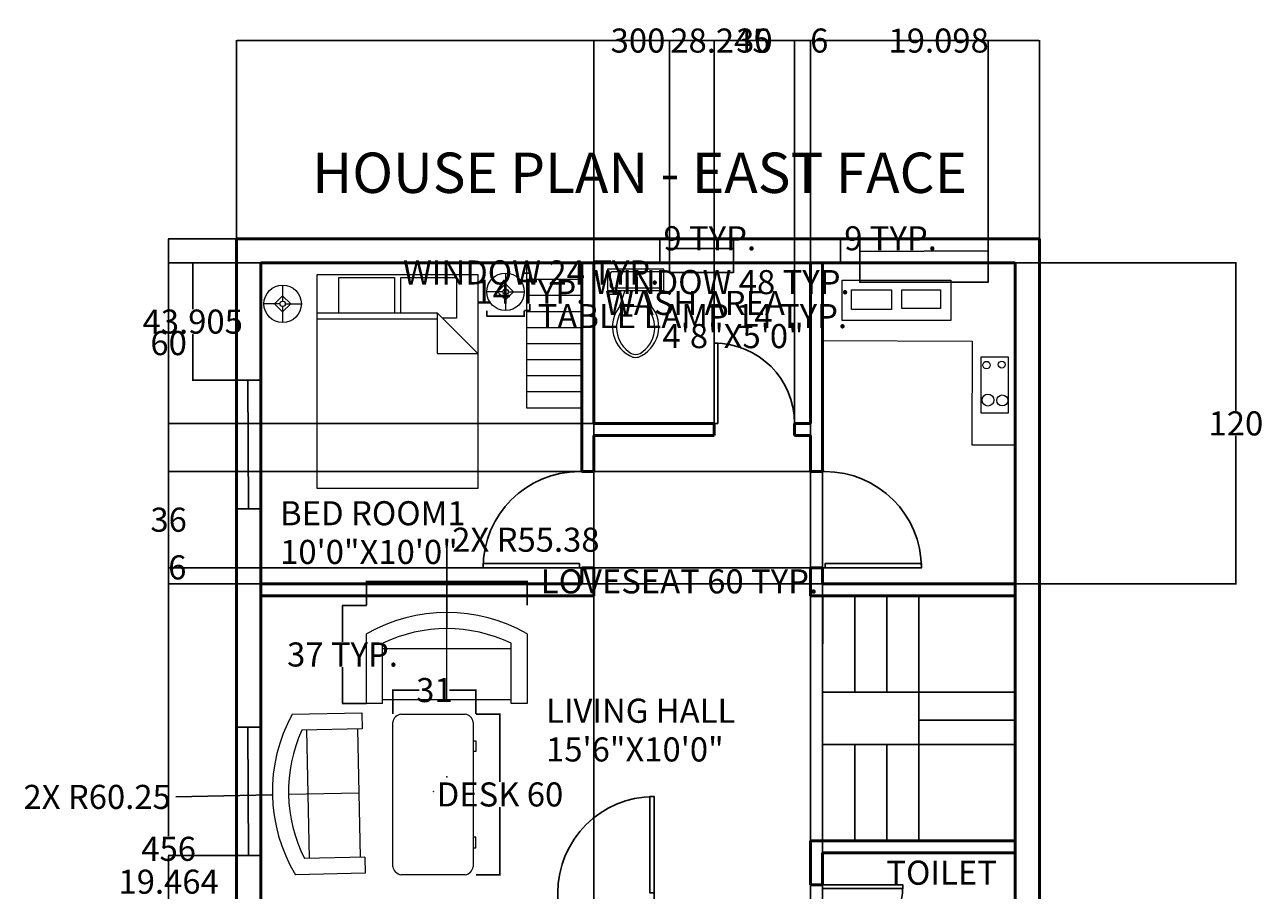
# Model space of a CAD drawing. Units: inches. Extents: x -49 to 419, y 83 to 650.
# Tile 2 of 2: x -49 to 414, y 327 to 650. Entities that reach past the tile are written whole.
import ezdxf

# ---------------------------------------------------------------- set-up
doc = ezdxf.new("R2010")
doc.units = ezdxf.units.IN
for name, color, linetype, lineweight in [('A-ANNO-DIMS', 2, 'Continuous', 18), ('A-ANNO-TEXT', 2, 'Continuous', 35), ('A-AREA-IDEN', 2, 'Continuous', 25), ('A-DOOR', 20, 'Continuous', 25), ('A-EQPM', 130, 'Continuous', 18), ('A-FLOR-CASE', 130, 'Continuous', 18), ('A-FLOR-FIXT', 130, 'Continuous', 18), ('A-FLOR-STRS', 150, 'Continuous', 25), ('A-GLAZ', 70, 'Continuous', 25), ('FUR', 130, 'Continuous', 18), ('WAL', 210, 'Continuous', 50)]:
    doc.layers.add(name, color=color, linetype=linetype, lineweight=lineweight)
doc.styles.get("Standard").update_dxf_attribs({"font": 'arial.ttf', "height": 9})
doc.dimstyles.get("Standard").update_dxf_attribs({"dimtxt": 0.18, "dimasz": 0.18, "dimexe": 0.18, "dimexo": 0.0625, "dimgap": 0.09, "dimtad": 0, "dimtih": 1, "dimtoh": 1, "dimdec": 4, "dimzin": 0, "dimdsep": 46, "dimtxsty": 'Standard', "dimcen": 0.09, "dimadec": 0, "dimazin": 0, "dimtfac": 1, "dimtdec": 4, "dimtofl": 0, "dimtmove": 0, "dimatfit": 3, "dimfxl": 1, "dimtolj": 1, "dimtzin": 0, "dimarcsym": 0})

# ---------------------------------------------------------------- blocks, each defined once
blk = doc.blocks.new('*U2')
for p, q in [((0, 0), (0, -6)), ((40, 0), (40, -6))]:
    blk.add_line(p, q)
blk.add_lwpolyline([(0, 0), (0, 40), (1.75, 40), (1.75, 0)], close=True)
blk.add_arc((0, 0), 40, 0, 90)
blk = doc.blocks.new('*U4')
for p, q in [((9.5, -6), (9.5, -2)), ((-10, -8.5), (-8, -8.5)), ((-10, -9.5), (-10, -8.5)), ((-8, -8.5), (-8, -8)), ((-7, -8), (-7, -9.5)), ((-4, -8), (-6, -14)), ((4, -8), (6, -14)), ((-7, -9.5), (-10, -9.5)), ((4, -14), (-4, -14))]:
    blk.add_line(p, q)
blk.add_lwpolyline([(10.5, -8), (10.5, 0), (-10.5, 0), (-10.5, -8)], close=True)
for points in [[(-9.5, -2), (-9.5, -6)], [(8.5, -1), (-8.5, -1)], [(-8.5, -7), (8.5, -7)]]:
    blk.add_lwpolyline(points)
for centre, radius, start, end in [((-8.62, -1.88), 0.884, 81.8699, 188.1301), ((8.62, -1.88), 0.884, 351.8699, 98.1301), ((-8.62, -6.12), 0.884, 171.8699, 278.1301), ((8.62, -6.12), 0.884, 261.8699, 8.1301), ((3.52, -21.58), 12.17, 141.4691, 247.9714), ((4.2, -21.82), 11.33, 136.3677, 238.9468), ((-3.52, -21.58), 12.17, 292.0284, 38.5307), ((-4.2, -21.82), 11.33, 301.053, 43.6321), ((0, -27.88), 4, 245.7318, 294.2682), ((0, -29), 4, 254.8605, 285.1395)]:
    blk.add_arc(centre, radius, start, end)
blk = doc.blocks.new('Bed - Queen')
for p, q in [((0, -80.00003), (0, 0)), ((0, 0), (59.99999, 0)), ((59.99999, 0), (59.99999, -80.00003)), ((7.99999, -1.2), (28.79998, -1.2)), ((7.99999, -14.4), (7.99999, -1.2)), ((28.79998, -1.2), (28.79998, -14.4)), ((31.19999, -1.2), (51.99999, -1.2)), ((31.19999, -14.4), (31.19999, -1.2)), ((51.99999, -1.2), (51.99999, -16.4)), ((0, -14.4), (44.8, -14.4)), ((44.8, -16.8), (0, -16.8)), ((59.99999, -29.6), (44.8, -14.4)), ((44.8, -14.4), (44.8, -29.6)), ((51.99999, -16.4), (46.79936, -16.4)), ((44.8, -29.6), (59.99999, -29.6)), ((59.99999, -80.00003), (0, -80.00003))]:
    blk.add_line(p, q)
blk = doc.blocks.new('Lamp - Table')
for p, q in [((0, 7), (0, 1)), ((-1, 0), (-7, 0)), ((0, 3), (-3, 0)), ((-3, 0), (0, -3)), ((3, 0), (0, 3)), ((0, -3), (3, 0)), ((1, 0), (7, 0)), ((0, -1), (0, -7))]:
    blk.add_line(p, q)
for radius in [7, 1]:
    blk.add_circle((0, 0), radius)
blk = doc.blocks.new('Desk - 30 x 60 in.')
for p, q in [((-26.999995, 0), (26.999995, 0)), ((-29.999995, -27), (-29.999995, -3)), ((29.999995, -3), (29.999995, -27)), ((26.999995, -30), (-26.999995, -30)), ((-20.000005, -30), (-20.000005, -31)), ((-20.000005, -31), (-16.000005, -31)), ((-16.000005, -31), (-16.000005, -30)), ((15.999995, -31), (15.999995, -30)), ((19.999995, -31), (15.999995, -31)), ((19.999995, -30), (19.999995, -31))]:
    blk.add_line(p, q)
for centre, start, end in [((-26.499995, -3.5), 98.1301, 171.8699), ((26.499995, -3.5), 8.130102, 81.8699), ((-26.499995, -26.5), 188.1301, 261.8699), ((26.499995, -26.5), 278.1301, 351.8699)]:
    blk.add_arc(centre, 3.535534, start, end)
blk = doc.blocks.new('Sofa - Roundback Loveseat 5 ft.')
for p, q in [((0, -32.44198), (0, -5.99998)), ((-24, -33.99998), (-24, -11.46958)), ((-23.9998, -13.38178), (23.99986, -13.38178)), ((24.00004, -33.99998), (24.00004, -11.46958)), ((-24, -32.44198), (24.00004, -32.44198))]:
    blk.add_line(p, q)
for points in [[(-24, -33.99998), (-30, -33.99998), (-30, -7.99998)], [(30.00004, -7.99998), (30.00004, -33.99998), (24.00004, -33.99998)]]:
    blk.add_lwpolyline(points)
for centre, radius, start, end in [((0, -60.24998), 60.24998, 60.13715, 119.8628), ((0, -61.38438), 55.38444, 64.32083, 115.6792)]:
    blk.add_arc(centre, radius, start, end)
blk = doc.blocks.new('WIN-48IN')
for p, q in [((0, 48), (0, 0)), ((9, 48), (0, 48)), ((4.19, 48), (4.5, 0)), ((9, 0), (9, 48)), ((0, 0), (9, 0))]:
    blk.add_line(p, q)
blk = doc.blocks.new('WIN-24IN')
for p, q in [((0, 24), (0, 0)), ((9, 24), (0, 24)), ((0, 24), (5.33, 24)), ((5.33, 24), (5.33, 0)), ((9, 0), (9, 24)), ((0, 0), (9, 0))]:
    blk.add_line(p, q)
blk = doc.blocks.new('*D14')
at = {"layer": 'A-ANNO-DIMS', "color": 0, "lineweight": -2, "transparency": 16777216}
for p, q in [((262.9, 560.94), (262.9, 553.62)), ((310.9, 560.94), (310.9, 553.62)), ((262.9, 553.8), (262.72, 553.8)), ((310.72, 553.8), (263.08, 553.8))]:
    blk.add_line(p, q, dxfattribs=at)
at = {"layer": 'A-ANNO-DIMS', "color": 0, "transparency": 16777216}
for points in [[(263.08, 553.83), (263.08, 553.77), (262.9, 553.8)], [(310.72, 553.83), (310.72, 553.77), (310.9, 553.8)]]:
    blk.add_solid(points, dxfattribs=at)
at = {"layer": 'Defpoints', "color": 0, "transparency": 16777216}
for p in [(262.9, 561), (310.9, 561), (262.9, 553.8)]:
    blk.add_point(p, dxfattribs=at)
at = {"layer": 'A-ANNO-DIMS', "color": 0, "transparency": 16777216, "insert": (211.21, 553.8), "char_height": 9, "attachment_point": 5}
blk.add_mtext('\\A1;WINDOW 48 TYP.', dxfattribs=at)
blk = doc.blocks.new('*D15')
at = {"layer": 'A-ANNO-DIMS', "color": 0, "lineweight": -2, "transparency": 16777216}
for p, q in [((262.84, 570), (255.52, 570)), ((255.7, 570), (255.7, 570.18)), ((255.7, 570.18), (255.88, 570.18)), ((255.7, 561.18), (255.7, 569.82)), ((262.84, 561), (255.52, 561))]:
    blk.add_line(p, q, dxfattribs=at)
at = {"layer": 'A-ANNO-DIMS', "color": 0, "transparency": 16777216}
for points in [[(255.67, 569.82), (255.73, 569.82), (255.7, 570)], [(255.67, 561.18), (255.73, 561.18), (255.7, 561)]]:
    blk.add_solid(points, dxfattribs=at)
at = {"layer": 'Defpoints', "color": 0, "transparency": 16777216}
for p in [(255.7, 570), (262.9, 570), (262.9, 561)]:
    blk.add_point(p, dxfattribs=at)
at = {"layer": 'A-ANNO-DIMS', "color": 0, "transparency": 16777216, "insert": (274.38, 570.18), "char_height": 9, "attachment_point": 5}
blk.add_mtext('\\A1;9 TYP.', dxfattribs=at)
blk = doc.blocks.new('*D16')
at = {"layer": 'A-ANNO-DIMS', "color": 0, "lineweight": -2, "transparency": 16777216}
for p, q in [((191.74, 560.94), (191.74, 557.22)), ((215.74, 560.94), (215.74, 557.22)), ((191.74, 557.4), (191.56, 557.4)), ((215.56, 557.4), (191.92, 557.4))]:
    blk.add_line(p, q, dxfattribs=at)
at = {"layer": 'A-ANNO-DIMS', "color": 0, "transparency": 16777216}
for points in [[(191.92, 557.43), (191.92, 557.37), (191.74, 557.4)], [(215.56, 557.43), (215.56, 557.37), (215.74, 557.4)]]:
    blk.add_solid(points, dxfattribs=at)
at = {"layer": 'Defpoints', "color": 0, "transparency": 16777216}
for p in [(191.74, 561), (215.74, 561), (191.74, 557.4)]:
    blk.add_point(p, dxfattribs=at)
at = {"layer": 'A-ANNO-DIMS', "color": 0, "transparency": 16777216, "insert": (140.06, 557.4), "char_height": 9, "attachment_point": 5}
blk.add_mtext('\\A1;WINDOW 24 TYP.', dxfattribs=at)
blk = doc.blocks.new('*D17')
at = {"layer": 'A-ANNO-DIMS', "color": 0, "lineweight": -2, "transparency": 16777216}
for p, q in [((191.68, 570), (187.96, 570)), ((188.14, 570), (188.14, 570.18)), ((188.14, 570.18), (188.32, 570.18)), ((188.14, 561.18), (188.14, 569.82)), ((191.68, 561), (187.96, 561))]:
    blk.add_line(p, q, dxfattribs=at)
at = {"layer": 'A-ANNO-DIMS', "color": 0, "transparency": 16777216}
for points in [[(188.11, 569.82), (188.17, 569.82), (188.14, 570)], [(188.11, 561.18), (188.17, 561.18), (188.14, 561)]]:
    blk.add_solid(points, dxfattribs=at)
at = {"layer": 'Defpoints', "color": 0, "transparency": 16777216}
for p in [(188.14, 570), (191.74, 570), (191.74, 561)]:
    blk.add_point(p, dxfattribs=at)
at = {"layer": 'A-ANNO-DIMS', "color": 0, "transparency": 16777216, "insert": (206.82, 570.18), "char_height": 9, "attachment_point": 5}
blk.add_mtext('\\A1;9 TYP.', dxfattribs=at)
blk = doc.blocks.new('*D20')
at = {"layer": 'A-ANNO-DIMS', "color": 0, "lineweight": -2, "transparency": 16777216}
for p, q in [((123.51, 543.12), (123.51, 540.91)), ((137.51, 543.12), (137.51, 540.91)), ((123.69, 541.09), (137.33, 541.09)), ((137.51, 541.09), (137.69, 541.09))]:
    blk.add_line(p, q, dxfattribs=at)
at = {"layer": 'A-ANNO-DIMS', "color": 0, "transparency": 16777216}
for points in [[(123.69, 541.12), (123.69, 541.06), (123.51, 541.09)], [(137.33, 541.12), (137.33, 541.06), (137.51, 541.09)]]:
    blk.add_solid(points, dxfattribs=at)
at = {"layer": 'Defpoints', "color": 0, "transparency": 16777216}
for p in [(123.51, 543.19), (137.51, 543.19), (137.51, 541.09)]:
    blk.add_point(p, dxfattribs=at)
at = {"layer": 'A-ANNO-DIMS', "color": 0, "transparency": 16777216, "insert": (200.33, 541.09), "char_height": 9, "attachment_point": 5}
blk.add_mtext('\\A1;TABLE LAMP 14 TYP.', dxfattribs=at)
blk = doc.blocks.new('*D21')
at = {"layer": 'A-ANNO-DIMS', "color": 0, "lineweight": -2, "transparency": 16777216}
for p, q in [((137.57, 557.19), (139.79, 557.19)), ((139.61, 557.01), (139.61, 554.8)), ((137.57, 543.19), (139.79, 543.19)), ((139.61, 543.37), (139.61, 545.57))]:
    blk.add_line(p, q, dxfattribs=at)
at = {"layer": 'A-ANNO-DIMS', "color": 0, "transparency": 16777216}
for points in [[(139.58, 557.01), (139.64, 557.01), (139.61, 557.19)], [(139.58, 543.37), (139.64, 543.37), (139.61, 543.19)]]:
    blk.add_solid(points, dxfattribs=at)
at = {"layer": 'Defpoints', "color": 0, "transparency": 16777216}
for p in [(137.51, 557.19), (139.61, 557.19), (137.51, 543.19)]:
    blk.add_point(p, dxfattribs=at)
at = {"layer": 'A-ANNO-DIMS', "color": 0, "transparency": 16777216, "insert": (139.61, 550.19), "char_height": 9, "attachment_point": 5}
blk.add_mtext('\\A1;14 TYP.', dxfattribs=at)
blk = doc.blocks.new('*D22')
at = {"layer": 'A-ANNO-DIMS', "color": 0, "lineweight": -2, "transparency": 16777216}
for p, q in [((78.58, 433.02), (78.58, 442.14)), ((78.76, 441.96), (138.4, 441.96)), ((138.58, 433.02), (138.58, 442.14)), ((138.58, 441.96), (138.76, 441.96))]:
    blk.add_line(p, q, dxfattribs=at)
at = {"layer": 'A-ANNO-DIMS', "color": 0, "transparency": 16777216}
for points in [[(78.76, 441.99), (78.76, 441.93), (78.58, 441.96)], [(138.4, 441.99), (138.4, 441.93), (138.58, 441.96)]]:
    blk.add_solid(points, dxfattribs=at)
at = {"layer": 'Defpoints', "color": 0, "transparency": 16777216}
for p in [(138.58, 441.96), (78.58, 432.96), (138.58, 432.96)]:
    blk.add_point(p, dxfattribs=at)
at = {"layer": 'A-ANNO-DIMS', "color": 0, "transparency": 16777216, "insert": (195.49, 441.96), "char_height": 9, "attachment_point": 5}
blk.add_mtext('\\A1;LOVESEAT 60 TYP.', dxfattribs=at)
blk = doc.blocks.new('*D23')
at = {"layer": 'A-ANNO-DIMS', "color": 0, "lineweight": -2, "transparency": 16777216}
for p, q in [((78.52, 432.96), (69.4, 432.96)), ((69.58, 432.78), (69.58, 419.32)), ((69.58, 396.48), (69.58, 409.94)), ((78.52, 396.3), (69.4, 396.3))]:
    blk.add_line(p, q, dxfattribs=at)
at = {"layer": 'A-ANNO-DIMS', "color": 0, "transparency": 16777216}
for points in [[(69.55, 432.78), (69.61, 432.78), (69.58, 432.96)], [(69.55, 396.48), (69.61, 396.48), (69.58, 396.3)]]:
    blk.add_solid(points, dxfattribs=at)
at = {"layer": 'Defpoints', "color": 0, "transparency": 16777216}
for p in [(69.58, 432.96), (78.58, 432.96), (78.58, 396.3)]:
    blk.add_point(p, dxfattribs=at)
at = {"layer": 'A-ANNO-DIMS', "color": 0, "transparency": 16777216, "insert": (69.58, 414.63), "char_height": 9, "attachment_point": 5}
blk.add_mtext('\\A1;37 TYP.', dxfattribs=at)
blk = doc.blocks.new('*D24')
at = {"layer": 'A-ANNO-DIMS', "color": 0, "lineweight": -2, "transparency": 16777216}
for p, q in [((119.49, 392.33), (128.6, 392.33)), ((128.42, 392.15), (128.42, 367.08)), ((128.42, 332.51), (128.42, 357.59)), ((119.49, 332.33), (128.6, 332.33))]:
    blk.add_line(p, q, dxfattribs=at)
at = {"layer": 'A-ANNO-DIMS', "color": 0, "transparency": 16777216}
for points in [[(128.39, 392.15), (128.45, 392.15), (128.42, 392.33)], [(128.39, 332.51), (128.45, 332.51), (128.42, 332.33)]]:
    blk.add_solid(points, dxfattribs=at)
at = {"layer": 'Defpoints', "color": 0, "transparency": 16777216}
for p in [(119.42, 392.33), (128.42, 392.33), (119.42, 332.33)]:
    blk.add_point(p, dxfattribs=at)
at = {"layer": 'A-ANNO-DIMS', "color": 0, "transparency": 16777216, "insert": (128.42, 362.33), "char_height": 9, "attachment_point": 5}
blk.add_mtext('\\A1;DESK 60', dxfattribs=at)
blk = doc.blocks.new('*D25')
at = {"layer": 'A-ANNO-DIMS', "color": 0, "lineweight": -2, "transparency": 16777216}
for p, q in [((88.42, 392.4), (88.42, 401.51)), ((88.6, 401.33), (98.26, 401.33)), ((119.24, 401.33), (109.59, 401.33)), ((119.42, 392.4), (119.42, 401.51))]:
    blk.add_line(p, q, dxfattribs=at)
at = {"layer": 'A-ANNO-DIMS', "color": 0, "transparency": 16777216}
for points in [[(88.6, 401.36), (88.6, 401.3), (88.42, 401.33)], [(119.24, 401.36), (119.24, 401.3), (119.42, 401.33)]]:
    blk.add_solid(points, dxfattribs=at)
at = {"layer": 'Defpoints', "color": 0, "transparency": 16777216}
for p in [(88.42, 401.33), (88.42, 392.33), (119.42, 392.33)]:
    blk.add_point(p, dxfattribs=at)
at = {"layer": 'A-ANNO-DIMS', "color": 0, "transparency": 16777216, "insert": (103.92, 401.33), "char_height": 9, "attachment_point": 5}
blk.add_mtext('\\A1;31', dxfattribs=at)
blk = doc.blocks.new('*D26')
at = {"layer": 'A-ANNO-DIMS', "color": 0, "lineweight": -2, "transparency": 16777216}
for p, q in [((30, 570.06), (30, 644.25)), ((30.18, 644.07), (169.99, 644.07)), ((329.82, 644.07), (190.01, 644.07)), ((330, 570.06), (330, 644.25))]:
    blk.add_line(p, q, dxfattribs=at)
at = {"layer": 'A-ANNO-DIMS', "color": 0, "transparency": 16777216}
for points in [[(30.18, 644.1), (30.18, 644.04), (30, 644.07)], [(329.82, 644.1), (329.82, 644.04), (330, 644.07)]]:
    blk.add_solid(points, dxfattribs=at)
at = {"layer": 'Defpoints', "color": 0, "transparency": 16777216}
for p in [(330, 644.07), (30, 570), (330, 570)]:
    blk.add_point(p, dxfattribs=at)
at = {"layer": 'A-ANNO-DIMS', "color": 0, "transparency": 16777216, "insert": (180, 644.07), "char_height": 9, "attachment_point": 5}
blk.add_mtext('\\A1;300', dxfattribs=at)
blk = doc.blocks.new('*D27')
at = {"layer": 'A-ANNO-DIMS', "color": 0, "lineweight": -2, "transparency": 16777216}
for p, q in [((29.94, 570), (4.42, 570)), ((4.6, 569.82), (4.6, 346.69)), ((4.6, 114.18), (4.6, 337.31)), ((29.94, 114), (4.42, 114))]:
    blk.add_line(p, q, dxfattribs=at)
at = {"layer": 'A-ANNO-DIMS', "color": 0, "transparency": 16777216}
for points in [[(4.57, 569.82), (4.63, 569.82), (4.6, 570)], [(4.57, 114.18), (4.63, 114.18), (4.6, 114)]]:
    blk.add_solid(points, dxfattribs=at)
at = {"layer": 'Defpoints', "color": 0, "transparency": 16777216}
for p in [(4.6, 570), (30, 570), (30, 114)]:
    blk.add_point(p, dxfattribs=at)
at = {"layer": 'A-ANNO-DIMS', "color": 0, "transparency": 16777216, "insert": (4.6, 342), "char_height": 9, "attachment_point": 5}
blk.add_mtext('\\A1;456', dxfattribs=at)
blk = doc.blocks.new('*D30')
at = {"layer": 'A-ANNO-DIMS', "color": 0, "lineweight": -2, "transparency": 16777216}
for p, q in [((29.94, 339.46), (4.42, 339.46)), ((4.6, 339.28), (4.6, 334.42)), ((4.6, 320.18), (4.6, 325.05)), ((38.94, 320), (4.42, 320))]:
    blk.add_line(p, q, dxfattribs=at)
at = {"layer": 'A-ANNO-DIMS', "color": 0, "transparency": 16777216}
for points in [[(4.57, 339.28), (4.63, 339.28), (4.6, 339.46)], [(4.57, 320.18), (4.63, 320.18), (4.6, 320)]]:
    blk.add_solid(points, dxfattribs=at)
at = {"layer": 'Defpoints', "color": 0, "transparency": 16777216}
for p in [(30, 339.46), (4.6, 320), (39, 320)]:
    blk.add_point(p, dxfattribs=at)
at = {"layer": 'A-ANNO-DIMS', "color": 0, "transparency": 16777216, "insert": (4.6, 329.73), "char_height": 9, "attachment_point": 5}
blk.add_mtext('\\A1;19.464', dxfattribs=at)
blk = doc.blocks.new('*D31')
at = {"layer": 'A-ANNO-DIMS', "color": 0, "lineweight": -2, "transparency": 16777216}
for p, q in [((38.94, 561), (13.42, 561)), ((13.6, 560.82), (13.6, 543.74)), ((13.6, 517.27), (13.6, 534.36)), ((38.94, 517.09), (13.42, 517.09))]:
    blk.add_line(p, q, dxfattribs=at)
at = {"layer": 'A-ANNO-DIMS', "color": 0, "transparency": 16777216}
for points in [[(13.57, 560.82), (13.63, 560.82), (13.6, 561)], [(13.57, 517.27), (13.63, 517.27), (13.6, 517.09)]]:
    blk.add_solid(points, dxfattribs=at)
at = {"layer": 'Defpoints', "color": 0, "transparency": 16777216}
for p in [(13.6, 561), (39, 561), (39, 517.09)]:
    blk.add_point(p, dxfattribs=at)
at = {"layer": 'A-ANNO-DIMS', "color": 0, "transparency": 16777216, "insert": (13.6, 539.05), "char_height": 9, "attachment_point": 5}
blk.add_mtext('\\A1;43.905', dxfattribs=at)
blk = doc.blocks.new('*D32')
at = {"layer": 'A-ANNO-DIMS', "color": 0, "lineweight": -2, "transparency": 16777216}
for p, q in [((163.5, 561.06), (163.5, 644.25)), ((163.68, 644.07), (191.56, 644.07)), ((191.74, 561.06), (191.74, 644.25)), ((191.74, 644.07), (191.92, 644.07))]:
    blk.add_line(p, q, dxfattribs=at)
at = {"layer": 'A-ANNO-DIMS', "color": 0, "transparency": 16777216}
for points in [[(163.68, 644.1), (163.68, 644.04), (163.5, 644.07)], [(191.56, 644.1), (191.56, 644.04), (191.74, 644.07)]]:
    blk.add_solid(points, dxfattribs=at)
at = {"layer": 'Defpoints', "color": 0, "transparency": 16777216}
for p in [(191.74, 644.07), (163.5, 561), (191.74, 561)]:
    blk.add_point(p, dxfattribs=at)
at = {"layer": 'A-ANNO-DIMS', "color": 0, "transparency": 16777216, "insert": (210.81, 644.07), "char_height": 9, "attachment_point": 5}
blk.add_mtext('\\A1;28.245', dxfattribs=at)
blk = doc.blocks.new('*D33')
at = {"layer": 'A-ANNO-DIMS', "color": 0, "lineweight": -2, "transparency": 16777216}
for p, q in [((310.9, 644.07), (310.72, 644.07)), ((310.9, 570.06), (310.9, 644.25)), ((329.82, 644.07), (311.08, 644.07)), ((330, 570.06), (330, 644.25))]:
    blk.add_line(p, q, dxfattribs=at)
at = {"layer": 'A-ANNO-DIMS', "color": 0, "transparency": 16777216}
for points in [[(311.08, 644.1), (311.08, 644.04), (310.9, 644.07)], [(329.82, 644.1), (329.82, 644.04), (330, 644.07)]]:
    blk.add_solid(points, dxfattribs=at)
at = {"layer": 'Defpoints', "color": 0, "transparency": 16777216}
for p in [(310.9, 644.07), (310.9, 570), (330, 570)]:
    blk.add_point(p, dxfattribs=at)
at = {"layer": 'A-ANNO-DIMS', "color": 0, "transparency": 16777216, "insert": (292.36, 644.07), "char_height": 9, "attachment_point": 5}
blk.add_mtext('\\A1;19.098', dxfattribs=at)
blk = doc.blocks.new('*D36')
at = {"layer": 'A-ANNO-DIMS', "color": 0, "lineweight": -2, "transparency": 16777216}
for p, q in [((163.5, 500.94), (163.5, 88.42)), ((244.5, 500.94), (244.5, 88.42)), ((163.68, 88.6), (198.33, 88.6)), ((244.32, 88.6), (209.67, 88.6))]:
    blk.add_line(p, q, dxfattribs=at)
at = {"layer": 'A-ANNO-DIMS', "color": 0, "transparency": 16777216}
for points in [[(163.68, 88.63), (163.68, 88.57), (163.5, 88.6)], [(244.32, 88.63), (244.32, 88.57), (244.5, 88.6)]]:
    blk.add_solid(points, dxfattribs=at)
at = {"layer": 'Defpoints', "color": 0, "transparency": 16777216}
for p in [(163.5, 501), (244.5, 501), (244.5, 88.6)]:
    blk.add_point(p, dxfattribs=at)
at = {"layer": 'A-ANNO-DIMS', "color": 0, "transparency": 16777216, "insert": (204, 88.6), "char_height": 9, "attachment_point": 5}
blk.add_mtext('\\A1;81', dxfattribs=at)
blk = doc.blocks.new('*D37')
at = {"layer": 'A-ANNO-DIMS', "color": 0, "lineweight": -2, "transparency": 16777216}
for p, q in [((249, 440.94), (249, 88.42)), ((321, 440.94), (321, 88.42)), ((249.18, 88.6), (278.55, 88.6)), ((320.82, 88.6), (291.45, 88.6))]:
    blk.add_line(p, q, dxfattribs=at)
at = {"layer": 'A-ANNO-DIMS', "color": 0, "transparency": 16777216}
for points in [[(249.18, 88.63), (249.18, 88.57), (249, 88.6)], [(320.82, 88.63), (320.82, 88.57), (321, 88.6)]]:
    blk.add_solid(points, dxfattribs=at)
at = {"layer": 'Defpoints', "color": 0, "transparency": 16777216}
for p in [(249, 441), (321, 441), (321, 88.6)]:
    blk.add_point(p, dxfattribs=at)
at = {"layer": 'A-ANNO-DIMS', "color": 0, "transparency": 16777216, "insert": (285, 88.6), "char_height": 9, "attachment_point": 5}
blk.add_mtext('\\A1;72', dxfattribs=at)
blk = doc.blocks.new('*D38')
at = {"layer": 'A-ANNO-DIMS', "color": 0, "lineweight": -2, "transparency": 16777216}
for p, q in [((321.06, 561), (403.62, 561)), ((403.44, 560.82), (403.44, 505.69)), ((403.44, 441.18), (403.44, 496.31)), ((321.06, 441), (403.62, 441))]:
    blk.add_line(p, q, dxfattribs=at)
at = {"layer": 'A-ANNO-DIMS', "color": 0, "transparency": 16777216}
for points in [[(403.41, 560.82), (403.47, 560.82), (403.44, 561)], [(403.41, 441.18), (403.47, 441.18), (403.44, 441)]]:
    blk.add_solid(points, dxfattribs=at)
at = {"layer": 'Defpoints', "color": 0, "transparency": 16777216}
for p in [(321, 561), (321, 441), (403.44, 441)]:
    blk.add_point(p, dxfattribs=at)
at = {"layer": 'A-ANNO-DIMS', "color": 0, "transparency": 16777216, "insert": (403.44, 501), "char_height": 9, "attachment_point": 5}
blk.add_mtext('\\A1;120', dxfattribs=at)
blk = doc.blocks.new('*D39')
at = {"layer": 'A-ANNO-DIMS', "color": 0, "lineweight": -2, "transparency": 16777216}
for p, q in [((163.44, 561), (4.42, 561)), ((4.6, 560.82), (4.6, 535.69)), ((4.6, 501.18), (4.6, 526.31)), ((163.44, 501), (4.42, 501))]:
    blk.add_line(p, q, dxfattribs=at)
at = {"layer": 'A-ANNO-DIMS', "color": 0, "transparency": 16777216}
for points in [[(4.57, 560.82), (4.63, 560.82), (4.6, 561)], [(4.57, 501.18), (4.63, 501.18), (4.6, 501)]]:
    blk.add_solid(points, dxfattribs=at)
at = {"layer": 'Defpoints', "color": 0, "transparency": 16777216}
for p in [(4.6, 561), (163.5, 561), (163.5, 501)]:
    blk.add_point(p, dxfattribs=at)
at = {"layer": 'A-ANNO-DIMS', "color": 0, "transparency": 16777216, "insert": (4.6, 531), "char_height": 9, "attachment_point": 5}
blk.add_mtext('\\A1;60', dxfattribs=at)
blk = doc.blocks.new('*D40')
at = {"layer": 'A-ANNO-DIMS', "color": 0, "lineweight": -2, "transparency": 16777216}
for p, q in [((208.5, 501.06), (208.5, 644.25)), ((208.68, 644.07), (216.98, 644.07)), ((238.32, 644.07), (230.02, 644.07)), ((238.5, 501.06), (238.5, 644.25))]:
    blk.add_line(p, q, dxfattribs=at)
at = {"layer": 'A-ANNO-DIMS', "color": 0, "transparency": 16777216}
for points in [[(208.68, 644.1), (208.68, 644.04), (208.5, 644.07)], [(238.32, 644.1), (238.32, 644.04), (238.5, 644.07)]]:
    blk.add_solid(points, dxfattribs=at)
at = {"layer": 'Defpoints', "color": 0, "transparency": 16777216}
for p in [(238.5, 644.07), (208.5, 501), (238.5, 501)]:
    blk.add_point(p, dxfattribs=at)
at = {"layer": 'A-ANNO-DIMS', "color": 0, "transparency": 16777216, "insert": (223.5, 644.07), "char_height": 9, "attachment_point": 5}
blk.add_mtext('\\A1;30', dxfattribs=at)
blk = doc.blocks.new('*D41')
at = {"layer": 'A-ANNO-DIMS', "color": 0, "lineweight": -2, "transparency": 16777216}
for p, q in [((238.5, 501.06), (238.5, 644.25)), ((238.68, 644.07), (244.32, 644.07)), ((244.5, 501.06), (244.5, 644.25)), ((244.5, 644.07), (244.68, 644.07))]:
    blk.add_line(p, q, dxfattribs=at)
at = {"layer": 'A-ANNO-DIMS', "color": 0, "transparency": 16777216}
for points in [[(238.68, 644.1), (238.68, 644.04), (238.5, 644.07)], [(244.32, 644.1), (244.32, 644.04), (244.5, 644.07)]]:
    blk.add_solid(points, dxfattribs=at)
at = {"layer": 'Defpoints', "color": 0, "transparency": 16777216}
for p in [(244.5, 644.07), (238.5, 501), (244.5, 501)]:
    blk.add_point(p, dxfattribs=at)
at = {"layer": 'A-ANNO-DIMS', "color": 0, "transparency": 16777216, "insert": (247.74, 644.07), "char_height": 9, "attachment_point": 5}
blk.add_mtext('\\A1;6', dxfattribs=at)
blk = doc.blocks.new('*D42')
at = {"layer": 'A-ANNO-DIMS', "color": 0, "lineweight": -2, "transparency": 16777216}
for p, q in [((248.94, 483), (4.42, 483)), ((4.6, 482.82), (4.6, 469.69)), ((4.6, 447.18), (4.6, 460.31)), ((248.94, 447), (4.42, 447))]:
    blk.add_line(p, q, dxfattribs=at)
at = {"layer": 'A-ANNO-DIMS', "color": 0, "transparency": 16777216}
for points in [[(4.57, 482.82), (4.63, 482.82), (4.6, 483)], [(4.57, 447.18), (4.63, 447.18), (4.6, 447)]]:
    blk.add_solid(points, dxfattribs=at)
at = {"layer": 'Defpoints', "color": 0, "transparency": 16777216}
for p in [(4.6, 483), (249, 483), (249, 447)]:
    blk.add_point(p, dxfattribs=at)
at = {"layer": 'A-ANNO-DIMS', "color": 0, "transparency": 16777216, "insert": (4.6, 465), "char_height": 9, "attachment_point": 5}
blk.add_mtext('\\A1;36', dxfattribs=at)
blk = doc.blocks.new('*D43')
at = {"layer": 'A-ANNO-DIMS', "color": 0, "lineweight": -2, "transparency": 16777216}
for p, q in [((248.94, 447), (4.42, 447)), ((4.6, 447), (4.6, 447.18)), ((4.6, 447.18), (4.78, 447.18)), ((4.6, 441.18), (4.6, 446.82)), ((248.94, 441), (4.42, 441))]:
    blk.add_line(p, q, dxfattribs=at)
at = {"layer": 'A-ANNO-DIMS', "color": 0, "transparency": 16777216}
for points in [[(4.57, 446.82), (4.63, 446.82), (4.6, 447)], [(4.57, 441.18), (4.63, 441.18), (4.6, 441)]]:
    blk.add_solid(points, dxfattribs=at)
at = {"layer": 'Defpoints', "color": 0, "transparency": 16777216}
for p in [(4.6, 447), (249, 447), (249, 441)]:
    blk.add_point(p, dxfattribs=at)
at = {"layer": 'A-ANNO-DIMS', "color": 0, "transparency": 16777216, "insert": (7.84, 447.18), "char_height": 9, "attachment_point": 5}
blk.add_mtext('\\A1;6', dxfattribs=at)
blk = doc.blocks.new('*D44')
at = {"layer": 'A-ANNO-DIMS', "color": 0, "lineweight": -2, "transparency": 16777216}
for p, q in [((244.5, 482.94), (244.5, 88.42)), ((249, 482.94), (249, 88.42)), ((244.68, 88.6), (248.82, 88.6)), ((249, 88.6), (249.18, 88.6))]:
    blk.add_line(p, q, dxfattribs=at)
at = {"layer": 'A-ANNO-DIMS', "color": 0, "transparency": 16777216}
for points in [[(244.68, 88.63), (244.68, 88.57), (244.5, 88.6)], [(248.82, 88.63), (248.82, 88.57), (249, 88.6)]]:
    blk.add_solid(points, dxfattribs=at)
at = {"layer": 'Defpoints', "color": 0, "transparency": 16777216}
for p in [(244.5, 483), (249, 483), (249, 88.6)]:
    blk.add_point(p, dxfattribs=at)
at = {"layer": 'A-ANNO-DIMS', "color": 0, "transparency": 16777216, "insert": (257.68, 88.6), "char_height": 9, "attachment_point": 5}
blk.add_mtext('\\A1;4.5', dxfattribs=at)
blk = doc.blocks.new('*D47')
at = {"layer": 'A-ANNO-DIMS', "color": 0, "lineweight": -2, "transparency": 16777216}
for p, q in [((7.24, 361.41), (43.2, 362.15)), ((103.52, 363.39), (103.7, 363.39)), ((103.61, 363.3), (103.61, 363.48))]:
    blk.add_line(p, q, dxfattribs=at)
at = {"layer": 'A-ANNO-DIMS', "color": 0, "transparency": 16777216}
blk.add_solid([(43.2, 362.18), (43.2, 362.12), (43.38, 362.15)], dxfattribs=at)
at = {"layer": 'Defpoints', "color": 0, "transparency": 16777216}
for p in [(43.38, 362.15), (103.61, 363.39)]:
    blk.add_point(p, dxfattribs=at)
at = {"layer": 'A-ANNO-DIMS', "color": 0, "transparency": 16777216, "insert": (-22.13, 361.41), "char_height": 9, "attachment_point": 5}
blk.add_mtext('\\A1;2X R60.25', dxfattribs=at)
blk = doc.blocks.new('*D48')
at = {"layer": 'A-ANNO-DIMS', "color": 0, "lineweight": -2, "transparency": 16777216}
for p, q in [((108.76, 457.53), (108.58, 457.53)), ((108.58, 457.53), (108.58, 424.48)), ((108.49, 368.91), (108.67, 368.91)), ((108.58, 368.82), (108.58, 369))]:
    blk.add_line(p, q, dxfattribs=at)
at = {"layer": 'A-ANNO-DIMS', "color": 0, "transparency": 16777216}
blk.add_solid([(108.55, 424.48), (108.61, 424.48), (108.58, 424.3)], dxfattribs=at)
at = {"layer": 'Defpoints', "color": 0, "transparency": 16777216}
for p in [(108.58, 424.3), (108.58, 368.91)]:
    blk.add_point(p, dxfattribs=at)
at = {"layer": 'A-ANNO-DIMS', "color": 0, "transparency": 16777216, "insert": (138.1, 457.53), "char_height": 9, "attachment_point": 5}
blk.add_mtext('\\A1;2X R55.38', dxfattribs=at)

msp = doc.modelspace()

# ---------------------------------------------------------------- linework, layer by layer
at = {"layer": 'A-EQPM'}
msp.add_lwpolyline([(308.1924, 525.9157), (318.31, 525.9157), (318.31, 504.8381), (308.1924, 504.8381)], close=True, dxfattribs=at)
for centre, radius in [((310.2398, 522.7634), 1.4142), ((315.9145, 522.9887), 1.2934), ((310.7907, 509.7097), 2.2164), ((316.1555, 509.5668), 2.06)]:
    msp.add_circle(centre, radius, dxfattribs=at)
at = {"layer": 'A-FLOR-CASE'}
for p, q in [((138.2988, 561), (138.2988, 506.871)), ((138.2988, 554.871), (159, 554.871)), ((138.2988, 548.871), (159, 548.871)), ((138.2988, 542.871), (159, 542.871)), ((138.2988, 536.871), (159, 536.871)), ((138.2988, 530.871), (159, 530.871)), ((249, 531.979), (304.9085, 531.7413)), ((304.9085, 531.7413), (304.7438, 492.9993)), ((138.2988, 524.871), (159, 524.871)), ((138.2988, 518.871), (159, 518.871)), ((138.2988, 512.871), (159, 512.871)), ((138.2988, 506.871), (159, 506.871)), ((304.7438, 492.9993), (321, 492.9993))]:
    msp.add_line(p, q, dxfattribs=at)
at = {"layer": 'A-FLOR-FIXT'}
for points in [[(256.2608, 554.4972), (296.9082, 554.4972), (296.9082, 539.4303), (256.2608, 539.4303)], [(259.7386, 550.9083), (274.7792, 550.9083), (274.7792, 543.5715), (259.7386, 543.5715)], [(278.569, 550.9083), (293.0175, 550.9083), (293.0175, 543.9857), (278.569, 543.9857)]]:
    msp.add_lwpolyline(points, close=True, dxfattribs=at)
at = {"layer": 'A-FLOR-STRS'}
for p, q in [((249, 400.5), (249.0179, 436.5)), ((261, 400.494), (261.0179, 436.494)), ((273, 400.4881), (273.0179, 436.4881)), ((321, 436.5), (285, 436.5)), ((285, 436.5), (285, 400.5)), ((285, 400.5), (249, 400.5)), ((285, 400.5), (321, 400.5)), ((285, 400.5), (285, 381)), ((285, 390.0621), (321, 390.0621)), ((285, 381), (249, 381)), ((249, 381), (249, 345)), ((261, 381), (261, 345)), ((273, 381), (273, 345)), ((285, 345), (285, 381)), ((285, 381), (321, 381))]:
    msp.add_line(p, q, dxfattribs=at)
at = {"layer": 'WAL'}
for p, q in [((30, 570), (30, 114)), ((330, 570), (30, 570)), ((330, 570), (330, 114)), ((39, 561), (39, 123)), ((321, 561), (39, 561)), ((159, 561), (159, 483)), ((163.5, 561), (163.5, 501)), ((244.5, 561), (244.5, 501)), ((249, 561), (249, 483)), ((321, 561), (321, 123)), ((208.5, 501), (163.5, 501)), ((208.5, 496.5), (208.5, 501)), ((244.5, 501), (238.5, 501)), ((244.5, 501), (238.5, 501)), ((238.5, 501), (238.5, 496.5)), ((208.5, 496.5), (163.5, 496.5)), ((163.5, 496.5), (163.5, 483)), ((244.5, 496.5), (238.5, 496.5)), ((244.5, 496.5), (244.5, 483)), ((159, 483), (163.5, 483)), ((244.5, 483), (249, 483)), ((163.5, 447), (159, 447)), ((159, 447), (159, 441)), ((163.5, 441), (163.5, 447)), ((163.5, 447), (163.5, 441)), ((249, 447), (244.5, 447)), ((244.5, 447), (244.5, 441)), ((249, 441), (249, 447)), ((249, 447), (249, 441)), ((159, 441), (39, 441)), ((163.5, 441), (163.5, 436.5)), ((244.5, 441), (244.5, 436.5)), ((321, 441), (249, 441)), ((321, 441), (321, 436.5)), ((163.5, 436.5), (39, 436.5)), ((249.0179, 436.5), (244.5, 436.5)), ((321, 436.5), (249.0179, 436.5)), ((321, 345), (244.5, 345)), ((244.5, 345), (244.5, 328.5)), ((321, 340.5), (249, 340.5)), ((249, 340.5), (249, 328.5)), ((244.5, 328.5), (249, 328.5))]:
    msp.add_line(p, q, dxfattribs=at)

# ---------------------------------------------------------------- block references
at = {"layer": 'A-DOOR'}
for p, xscale, yscale, zscale in [((208.5, 501), 0.75, 0.75, 0.75), ((186, 325.5224), -0.9, 0.9, 0.9)]:
    msp.add_blockref('*U2', p, dxfattribs=dict(at, xscale=xscale, yscale=yscale, zscale=zscale))
for p, xscale, yscale, zscale, rotation in [((158.1, 447), 0.9, 0.9, 0.9, 90.00000000000003), ((249.9, 447), -0.9, 0.9, 0.9, 270), ((249, 328.5), 0.75, 0.75, 0.75, 270)]:
    msp.add_blockref('*U2', p, dxfattribs=dict(at, xscale=xscale, yscale=yscale, zscale=zscale, rotation=rotation))
at = {"layer": 'A-FLOR-FIXT'}
msp.add_blockref('*U4', (179.1067, 558.6666), dxfattribs=at)
at = {"layer": 'A-GLAZ'}
for name, p, rotation in [('WIN-24IN', (215.7444, 561), 90), ('WIN-48IN', (310.9018, 561), 89.99999999999987)]:
    msp.add_blockref(name, p, dxfattribs=dict(at, rotation=rotation))
for p in [(30, 469.0948), (30, 339.464)]:
    msp.add_blockref('WIN-48IN', p, dxfattribs=at)
at = {"layer": 'FUR'}
for name, p in [('Bed - Queen', (60.151, 556.6989)), ('Lamp - Table', (130.512, 550.1856)), ('Lamp - Table', (47.2019, 545.6855)), ('Sofa - Roundback Loveseat 5 ft.', (108.5809, 430.2951))]:
    msp.add_blockref(name, p, dxfattribs=at)
for name, p, rotation in [('Sofa - Roundback Loveseat 5 ft.', (43.3776, 362.1521), 91.18074240512688), ('Desk - 30 x 60 in.', (88.424, 362.3344), 90)]:
    msp.add_blockref(name, p, dxfattribs=dict(at, rotation=rotation))

# ---------------------------------------------------------------- texts
at = {"layer": 'A-ANNO-TEXT'}
msp.add_text('HOUSE PLAN - EAST FACE ', height=15.067584, dxfattribs=at).set_placement((58.2611, 587.1214))
at = {"layer": 'A-AREA-IDEN'}
for s, p in [('WASH AREA', (167.6848, 541.5222)), ('4\'8"X5\'0"', (189.1546, 529.1216)), ('BED ROOM1', (46.2581, 462.9198)), ('10\'0"X10\'0"', (46.2581, 448.4621)), ('LIVING HALL', (145.6313, 389.1045)), ('15\'6"X10\'0"', (145.6313, 374.6468)), ('TOILET', (272.822, 328.5903))]:
    msp.add_text(s, height=9, dxfattribs=at).set_placement(p)

# ---------------------------------------------------------------- dimensions: what is measured, and where the dimension line sits
at = {"layer": 'A-ANNO-DIMS'}
for base, p1, p2, override, picture, middle in [((330, 644.0666), (30, 570), (330, 570), {"dimdec": 0, "dimlfac": 1, "dimrnd": 0, "dimzin": 0, "dimdsep": 46, "dimlunit": 2}, '*D26', (180, 644.0666)), ((191.7448, 644.0666), (163.5, 561), (191.7448, 561), {"dimdec": 3, "dimlfac": 1, "dimrnd": 0, "dimzin": 0, "dimdsep": 46, "dimlunit": 2}, '*D32', (210.8067, 644.0666)), ((238.5, 644.0666), (208.5, 501), (238.5, 501), {"dimdec": 0, "dimlfac": 1, "dimrnd": 0, "dimzin": 0, "dimdsep": 46, "dimlunit": 2}, '*D40', (223.5, 644.0666)), ((244.5, 644.0666), (238.5, 501), (244.5, 501), {"dimdec": 0, "dimlfac": 1, "dimrnd": 0, "dimzin": 0, "dimdsep": 46, "dimlunit": 2}, '*D41', (247.7414, 644.0666)), ((310.902, 644.0666), (330, 570), (310.902, 570), {"dimdec": 3, "dimlfac": 1, "dimrnd": 0, "dimzin": 0, "dimdsep": 46, "dimlunit": 2}, '*D33', (292.365, 644.0666)), ((244.5, 88.6), (163.5, 501), (244.5, 501), {"dimdec": 0, "dimlfac": 1, "dimrnd": 0, "dimzin": 0, "dimdsep": 46, "dimlunit": 2}, '*D36', (204, 88.6)), ((249, 88.6), (244.5, 483), (249, 483), {"dimdec": 1, "dimlfac": 1, "dimrnd": 0, "dimzin": 0, "dimdsep": 46, "dimlunit": 2}, '*D44', (257.6776, 88.6)), ((321, 88.6), (249, 441), (321, 441), {"dimdec": 0, "dimlfac": 1, "dimrnd": 0, "dimzin": 0, "dimdsep": 46, "dimlunit": 2}, '*D37', (285, 88.6))]:
    dim = msp.add_linear_dim(base=base, p1=p1, p2=p2, dimstyle='Standard', override=override, dxfattribs=at)
    dim.commit()
    dim.dimension.update_dxf_attribs({"geometry": picture, "text_midpoint": middle})
for base, p1, p2, angle, text, picture, middle in [((188.1448, 570), (191.7448, 561), (191.7448, 570), 90, '<> TYP.', '*D17', (206.823, 570.18)), ((255.702, 570), (262.902, 561), (262.902, 570), 90, '<> TYP.', '*D15', (274.3803, 570.18)), ((191.7448, 557.4), (215.7448, 561), (191.7448, 561), 180, 'WINDOW <> TYP.', '*D16', (140.0563, 557.4)), ((262.902, 553.8), (310.902, 561), (262.902, 561), 180, 'WINDOW <> TYP.', '*D14', (211.2136, 553.8)), ((139.612, 557.1856), (137.512, 543.1856), (137.512, 557.1856), 90, '<> TYP.', '*D21', (139.612, 550.1856)), ((69.5809, 432.9618), (78.5809, 396.2951), (78.5809, 432.9618), 90, '<> TYP.', '*D23', (69.5809, 414.6285)), ((128.424, 392.3343), (119.424, 332.3344), (119.424, 392.3343), 90, 'DESK <>', '*D24', (128.424, 362.3344))]:
    dim = msp.add_linear_dim(base=base, p1=p1, p2=p2, angle=angle, text=text, dimstyle='Standard', override={"dimdec": 0, "dimlfac": 1, "dimrnd": 0, "dimzin": 0, "dimdsep": 46, "dimlunit": 2}, dxfattribs=at)
    dim.commit()
    dim.dimension.update_dxf_attribs({"geometry": picture, "text_midpoint": middle})
for base, p1, p2, angle, override, picture, middle in [((4.6, 570), (30, 114), (30, 570), 90, {"dimdec": 0, "dimlfac": 1, "dimrnd": 0, "dimzin": 0, "dimdsep": 46, "dimlunit": 2}, '*D27', (4.6, 342)), ((13.6, 561), (39, 517.09455), (39, 561), 90, {"dimdec": 3, "dimlfac": 1, "dimrnd": 0, "dimzin": 0, "dimdsep": 46, "dimlunit": 2}, '*D31', (13.6, 539.04727)), ((4.6, 561), (163.5, 501), (163.5, 561), 90, {"dimdec": 0, "dimlfac": 1, "dimrnd": 0, "dimzin": 0, "dimdsep": 46, "dimlunit": 2}, '*D39', (4.6, 531)), ((403.4356, 441), (321, 561), (321, 441), 90, {"dimdec": 0, "dimlfac": 1, "dimrnd": 0, "dimzin": 0, "dimdsep": 46, "dimlunit": 2}, '*D38', (403.4356, 501)), ((4.6, 483), (249, 447), (249, 483), 90, {"dimdec": 0, "dimlfac": 1, "dimrnd": 0, "dimzin": 0, "dimdsep": 46, "dimlunit": 2}, '*D42', (4.6, 465)), ((4.6, 447), (249, 441), (249, 447), 90, {"dimdec": 0, "dimlfac": 1, "dimrnd": 0, "dimzin": 0, "dimdsep": 46, "dimlunit": 2}, '*D43', (7.8414, 447.18)), ((88.424, 401.3343), (119.424, 392.3343), (88.424, 392.3343), 180, {"dimdec": 0, "dimlfac": 1, "dimrnd": 0, "dimzin": 0, "dimdsep": 46, "dimlunit": 2}, '*D25', (103.924, 401.3343)), ((4.6, 320), (30, 339.4638), (39, 320), 90, {"dimdec": 3, "dimlfac": 1, "dimrnd": 0, "dimzin": 0, "dimdsep": 46, "dimlunit": 2}, '*D30', (4.6, 329.7319))]:
    dim = msp.add_linear_dim(base=base, p1=p1, p2=p2, angle=angle, dimstyle='Standard', override=override, dxfattribs=at)
    dim.commit()
    dim.dimension.update_dxf_attribs({"geometry": picture, "text_midpoint": middle})
for base, p1, p2, text, picture, middle in [((137.512, 541.0856), (123.512, 543.1856), (137.512, 543.1856), 'TABLE LAMP <> TYP.', '*D20', (200.3277, 541.0856)), ((138.5809, 441.9618), (78.5809, 432.9618), (138.5809, 432.9618), 'LOVESEAT <> TYP.', '*D22', (195.4938, 441.9618))]:
    dim = msp.add_linear_dim(base=base, p1=p1, p2=p2, text=text, dimstyle='Standard', override={"dimdec": 0, "dimlfac": 1, "dimrnd": 0, "dimzin": 0, "dimdsep": 46, "dimlunit": 2}, dxfattribs=at)
    dim.commit()
    dim.dimension.update_dxf_attribs({"geometry": picture, "text_midpoint": middle})
for center, mpoint, picture, middle in [((108.5809, 368.9107), (108.581, 424.2952), '*D48', (138.098, 457.5258)), ((103.6147, 363.3936), (43.3776, 362.152), '*D47', (7.2352, 361.407))]:
    dim = msp.add_radius_dim(center=center, mpoint=mpoint, text='2X <>', dimstyle='Standard', override={"dimdec": 2, "dimlfac": 1, "dimrnd": 0, "dimzin": 0, "dimdsep": 46, "dimlunit": 2}, dxfattribs=at)
    dim.commit()
    dim.dimension.update_dxf_attribs({"geometry": picture, "text_midpoint": middle, "dimtype": 164})

doc.saveas('drawing.dxf')
